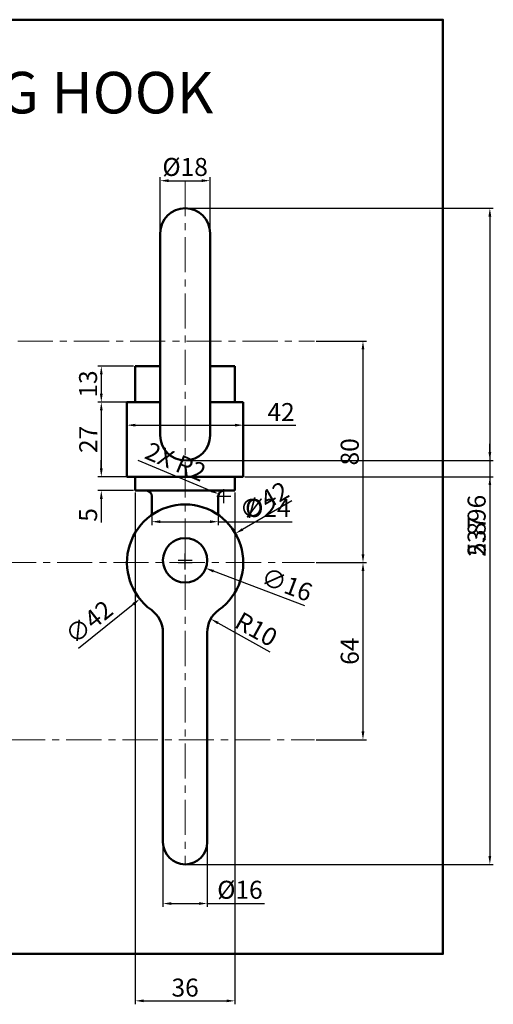
# Model space of a CAD drawing. Units: millimetres. Extents: x 309 to 670, y -17 to 339.
# Tile 2 of 2: x 498 to 670, y -17 to 339. Entities that reach past the tile are written whole.
import ezdxf

# ---------------------------------------------------------------- set-up
doc = ezdxf.new("R2010")
doc.units = ezdxf.units.MM
doc.header["$LTSCALE"] = 0.4
doc.linetypes.add('CENTER', pattern=[50.8, 31.75, -6.35, 6.35, -6.35])
for name, color, linetype, lineweight in [('M-CNTR', 1, 'CENTER', 18), ('M-DIMS', 2, 'Continuous', 25), ('M-OUTL', 7, 'Continuous', 50), ('M-TEXT', 7, 'Continuous', 25), ('M-TTLB', 7, 'Continuous', 50)]:
    doc.layers.add(name, color=color, linetype=linetype, lineweight=lineweight)
doc.styles.get("Standard").update_dxf_attribs({"font": 'arial.ttf'})
doc.dimstyles.new('ISO-25', dxfattribs={"dimtxt": 6.5, "dimasz": 3, "dimexe": 1.25, "dimexo": 0.625, "dimtad": 1, "dimdec": 0, "dimtxsty": 'Standard', "dimcen": 2.5, "dimadec": 0, "dimazin": 0, "dimtfac": 1, "dimtdec": 0, "dimtofl": 0, "dimtmove": 0, "dimatfit": 3, "dimfxl": 1, "dimarcsym": 0})

# ---------------------------------------------------------------- blocks, each defined once
blk = doc.blocks.new('*D1')
at = {"layer": 'Defpoints', "color": 0, "ltscale": 0.4, "transparency": 16777216}
for p in [(540.21, 213.66), (527.93, 200.66), (540.21, 200.66)]:
    blk.add_point(p, dxfattribs=at)
at = {"layer": 'M-DIMS', "color": 0, "lineweight": -2, "ltscale": 0.4, "transparency": 16777216}
for p, q in [((539.58, 213.66), (526.68, 213.66)), ((527.93, 210.66), (527.93, 203.66)), ((539.58, 200.66), (526.68, 200.66))]:
    blk.add_line(p, q, dxfattribs=at)
at = {"layer": 'M-DIMS', "color": 0, "ltscale": 0.4, "transparency": 16777216}
for points in [[(527.43, 210.66), (528.43, 210.66), (527.93, 213.66)], [(527.43, 203.66), (528.43, 203.66), (527.93, 200.66)]]:
    blk.add_solid(points, dxfattribs=at)
at = {"layer": 'M-DIMS', "color": 0, "ltscale": 0.4, "transparency": 16777216, "insert": (523.99, 207.16), "char_height": 6.5, "attachment_point": 5, "rotation": 90}
blk.add_mtext('13', dxfattribs=at)
blk = doc.blocks.new('*D2')
at = {"layer": 'Defpoints', "color": 0, "ltscale": 0.4, "transparency": 16777216}
for p in [(537.21, 200.66), (527.93, 173.66), (537.21, 173.66)]:
    blk.add_point(p, dxfattribs=at)
at = {"layer": 'M-DIMS', "color": 0, "lineweight": -2, "ltscale": 0.4, "transparency": 16777216}
for p, q in [((536.58, 200.66), (526.68, 200.66)), ((527.93, 197.66), (527.93, 176.66)), ((536.58, 173.66), (526.68, 173.66))]:
    blk.add_line(p, q, dxfattribs=at)
at = {"layer": 'M-DIMS', "color": 0, "ltscale": 0.4, "transparency": 16777216}
for points in [[(527.43, 197.66), (528.43, 197.66), (527.93, 200.66)], [(527.43, 176.66), (528.43, 176.66), (527.93, 173.66)]]:
    blk.add_solid(points, dxfattribs=at)
at = {"layer": 'M-DIMS', "color": 0, "ltscale": 0.4, "transparency": 16777216, "insert": (524.05, 187.16), "char_height": 6.5, "attachment_point": 5, "rotation": 90}
blk.add_mtext('27', dxfattribs=at)
blk = doc.blocks.new('*D3')
at = {"layer": 'Defpoints', "color": 0, "ltscale": 0.4, "transparency": 16777216}
for p in [(540.21, 173.66), (527.93, 168.66), (540.21, 168.66)]:
    blk.add_point(p, dxfattribs=at)
at = {"layer": 'M-DIMS', "color": 0, "lineweight": -2, "ltscale": 0.4, "transparency": 16777216}
for p, q in [((527.93, 176.66), (527.93, 179.66)), ((539.58, 173.66), (526.68, 173.66)), ((539.58, 168.66), (526.68, 168.66)), ((527.93, 165.66), (527.93, 157.1))]:
    blk.add_line(p, q, dxfattribs=at)
at = {"layer": 'M-DIMS', "color": 0, "ltscale": 0.4, "transparency": 16777216}
for points in [[(527.43, 176.66), (528.43, 176.66), (527.93, 173.66)], [(527.43, 165.66), (528.43, 165.66), (527.93, 168.66)]]:
    blk.add_solid(points, dxfattribs=at)
at = {"layer": 'M-DIMS', "color": 0, "ltscale": 0.4, "transparency": 16777216, "insert": (524, 159.88), "char_height": 6.5, "attachment_point": 5, "rotation": 90}
blk.add_mtext('5', dxfattribs=at)
blk = doc.blocks.new('*D4')
at = {"layer": 'Defpoints', "color": 0, "ltscale": 0.4, "transparency": 16777216}
for p in [(579.21, 192.3), (537.21, 180.61), (579.21, 180.61)]:
    blk.add_point(p, dxfattribs=at)
at = {"layer": 'M-DIMS', "color": 0, "lineweight": -2, "ltscale": 0.4, "transparency": 16777216}
for p, q in [((537.21, 181.24), (537.21, 193.55)), ((540.21, 192.3), (576.21, 192.3)), ((579.21, 181.24), (579.21, 193.55)), ((579.21, 192.3), (598.25, 192.3))]:
    blk.add_line(p, q, dxfattribs=at)
at = {"layer": 'M-DIMS', "color": 0, "ltscale": 0.4, "transparency": 16777216}
for points in [[(540.21, 192.8), (540.21, 191.8), (537.21, 192.3)], [(576.21, 192.8), (576.21, 191.8), (579.21, 192.3)]]:
    blk.add_solid(points, dxfattribs=at)
at = {"layer": 'M-DIMS', "color": 0, "ltscale": 0.4, "transparency": 16777216, "insert": (592.87, 196.19), "char_height": 6.5, "attachment_point": 5}
blk.add_mtext('42', dxfattribs=at)
blk = doc.blocks.new('*D5')
at = {"layer": 'Defpoints', "color": 0, "ltscale": 0.4, "transparency": 16777216}
for p in [(546.21, 159.89), (570.21, 159.89), (570.21, 157.43)]:
    blk.add_point(p, dxfattribs=at)
at = {"layer": 'M-DIMS', "color": 0, "lineweight": -2, "ltscale": 0.4, "transparency": 16777216}
for p, q in [((546.21, 159.26), (546.21, 156.18)), ((549.21, 157.43), (567.21, 157.43)), ((570.21, 159.26), (570.21, 156.18)), ((570.21, 157.43), (596.93, 157.43))]:
    blk.add_line(p, q, dxfattribs=at)
at = {"layer": 'M-DIMS', "color": 0, "ltscale": 0.4, "transparency": 16777216}
for points in [[(549.21, 157.93), (549.21, 156.93), (546.21, 157.43)], [(567.21, 157.93), (567.21, 156.93), (570.21, 157.43)]]:
    blk.add_solid(points, dxfattribs=at)
at = {"layer": 'M-DIMS', "color": 0, "ltscale": 0.4, "transparency": 16777216, "insert": (588.12, 161.55), "char_height": 6.5, "attachment_point": 5}
blk.add_mtext('%%C24', dxfattribs=at)
blk = doc.blocks.new('*D6')
at = {"layer": 'Defpoints', "color": 0, "ltscale": 0.4, "transparency": 16777216}
for p in [(567.21, 280.61), (549.21, 247.25), (567.21, 247.25)]:
    blk.add_point(p, dxfattribs=at)
at = {"layer": 'M-DIMS', "color": 0, "lineweight": -2, "ltscale": 0.4, "transparency": 16777216}
for p, q in [((549.21, 247.87), (549.21, 281.86)), ((567.21, 247.87), (567.21, 281.86)), ((552.21, 280.61), (564.21, 280.61))]:
    blk.add_line(p, q, dxfattribs=at)
at = {"layer": 'M-DIMS', "color": 0, "ltscale": 0.4, "transparency": 16777216}
for points in [[(552.21, 281.11), (552.21, 280.11), (549.21, 280.61)], [(564.21, 281.11), (564.21, 280.11), (567.21, 280.61)]]:
    blk.add_solid(points, dxfattribs=at)
at = {"layer": 'M-DIMS', "color": 0, "ltscale": 0.4, "transparency": 16777216, "insert": (558.21, 284.73), "char_height": 6.5, "attachment_point": 5}
blk.add_mtext('%%C18', dxfattribs=at)
blk = doc.blocks.new('*D7')
at = {"layer": 'Defpoints', "color": 0, "ltscale": 0.4, "transparency": 16777216}
for p in [(604.93, 222.66), (604.93, 142.66), (622.48, 142.66)]:
    blk.add_point(p, dxfattribs=at)
at = {"layer": 'M-DIMS', "color": 0, "lineweight": -2, "ltscale": 0.4, "transparency": 16777216}
for p, q in [((605.56, 222.66), (623.73, 222.66)), ((622.48, 219.66), (622.48, 145.66)), ((605.56, 142.66), (623.73, 142.66))]:
    blk.add_line(p, q, dxfattribs=at)
at = {"layer": 'M-DIMS', "color": 0, "ltscale": 0.4, "transparency": 16777216}
for points in [[(621.98, 219.66), (622.98, 219.66), (622.48, 222.66)], [(621.98, 145.66), (622.98, 145.66), (622.48, 142.66)]]:
    blk.add_solid(points, dxfattribs=at)
at = {"layer": 'M-DIMS', "color": 0, "ltscale": 0.4, "transparency": 16777216, "insert": (618.53, 182.66), "char_height": 6.5, "attachment_point": 5, "rotation": 90}
blk.add_mtext('80', dxfattribs=at)
blk = doc.blocks.new('*D8')
at = {"layer": 'Defpoints', "color": 0, "ltscale": 0.4, "transparency": 16777216}
for p in [(604.93, 142.66), (604.93, 78.66), (622.48, 78.66)]:
    blk.add_point(p, dxfattribs=at)
at = {"layer": 'M-DIMS', "color": 0, "lineweight": -2, "ltscale": 0.4, "transparency": 16777216}
for p, q in [((605.56, 142.66), (623.73, 142.66)), ((622.48, 139.66), (622.48, 81.66)), ((605.56, 78.66), (623.73, 78.66))]:
    blk.add_line(p, q, dxfattribs=at)
at = {"layer": 'M-DIMS', "color": 0, "ltscale": 0.4, "transparency": 16777216}
for points in [[(621.98, 139.66), (622.98, 139.66), (622.48, 142.66)], [(621.98, 81.66), (622.98, 81.66), (622.48, 78.66)]]:
    blk.add_solid(points, dxfattribs=at)
at = {"layer": 'M-DIMS', "color": 0, "ltscale": 0.4, "transparency": 16777216, "insert": (618.53, 110.66), "char_height": 6.5, "attachment_point": 5, "rotation": 90}
blk.add_mtext('64', dxfattribs=at)
blk = doc.blocks.new('*D9')
at = {"layer": 'Defpoints', "color": 0, "ltscale": 0.4, "transparency": 16777216}
for p in [(550.21, 50.97), (566.21, 50.97), (566.21, 19.51)]:
    blk.add_point(p, dxfattribs=at)
at = {"layer": 'M-DIMS', "color": 0, "lineweight": -2, "ltscale": 0.4, "transparency": 16777216}
for p, q in [((550.21, 50.35), (550.21, 18.26)), ((566.21, 50.35), (566.21, 18.26)), ((553.21, 19.51), (563.21, 19.51)), ((566.21, 19.51), (586.84, 19.51))]:
    blk.add_line(p, q, dxfattribs=at)
at = {"layer": 'M-DIMS', "color": 0, "ltscale": 0.4, "transparency": 16777216}
for points in [[(553.21, 20.01), (553.21, 19.01), (550.21, 19.51)], [(563.21, 20.01), (563.21, 19.01), (566.21, 19.51)]]:
    blk.add_solid(points, dxfattribs=at)
at = {"layer": 'M-DIMS', "color": 0, "ltscale": 0.4, "transparency": 16777216, "insert": (578.02, 23.64), "char_height": 6.5, "attachment_point": 5}
blk.add_mtext('%%C16', dxfattribs=at)
blk = doc.blocks.new('*D10')
at = {"layer": 'Defpoints', "color": 0, "ltscale": 0.4, "transparency": 16777216}
for p in [(567.48, 122.3), (576.21, 117.42)]:
    blk.add_point(p, dxfattribs=at)
at = {"layer": 'M-DIMS', "color": 0, "lineweight": -2, "ltscale": 0.4, "transparency": 16777216}
blk.add_line((588.9, 110.31), (570.1, 120.84), dxfattribs=at)
at = {"layer": 'M-DIMS', "color": 0, "ltscale": 0.4, "transparency": 16777216}
blk.add_solid([(570.34, 121.27), (569.85, 120.4), (567.48, 122.3)], dxfattribs=at)
at = {"layer": 'M-DIMS', "color": 0, "ltscale": 0.4, "transparency": 16777216, "insert": (583.52, 117.85), "char_height": 6.5, "attachment_point": 5, "rotation": 330.7676}
blk.add_mtext('R10', dxfattribs=at)
blk = doc.blocks.new('*D11')
at = {"layer": 'Defpoints', "color": 0, "ltscale": 0.4, "transparency": 16777216}
for p in [(574.59, 155.8), (541.83, 129.51)]:
    blk.add_point(p, dxfattribs=at)
at = {"layer": 'M-DIMS', "color": 0, "lineweight": -2, "ltscale": 0.4, "transparency": 16777216}
for p, q in [((555.71, 142.66), (560.71, 142.66)), ((558.21, 140.16), (558.21, 145.16)), ((519.73, 111.79), (539.49, 127.64))]:
    blk.add_line(p, q, dxfattribs=at)
at = {"layer": 'M-DIMS', "color": 0, "ltscale": 0.4, "transparency": 16777216}
blk.add_solid([(539.17, 128.03), (539.8, 127.25), (541.83, 129.51)], dxfattribs=at)
at = {"layer": 'M-DIMS', "color": 0, "ltscale": 0.4, "transparency": 16777216, "insert": (524, 120.5), "char_height": 6.5, "attachment_point": 5, "rotation": 38.7396}
blk.add_mtext('∅42', dxfattribs=at)
blk = doc.blocks.new('*D12')
at = {"layer": 'Defpoints', "color": 0, "ltscale": 0.4, "transparency": 16777216}
for p in [(550.73, 146.33), (565.68, 140.63)]:
    blk.add_point(p, dxfattribs=at)
at = {"layer": 'M-DIMS', "color": 0, "lineweight": -2, "ltscale": 0.4, "transparency": 16777216}
for p, q in [((558.21, 140.98), (558.21, 145.98)), ((555.71, 143.48), (560.71, 143.48)), ((601.46, 127), (568.49, 139.57))]:
    blk.add_line(p, q, dxfattribs=at)
at = {"layer": 'M-DIMS', "color": 0, "ltscale": 0.4, "transparency": 16777216}
blk.add_solid([(568.66, 140.03), (568.31, 139.1), (565.68, 140.63)], dxfattribs=at)
at = {"layer": 'M-DIMS', "color": 0, "ltscale": 0.4, "transparency": 16777216, "insert": (594.69, 133.99), "char_height": 6.5, "attachment_point": 5, "rotation": 339.135}
blk.add_mtext('∅16', dxfattribs=at)
blk = doc.blocks.new('*D29')
at = {"layer": 'Defpoints', "color": 0, "ltscale": 0.4, "transparency": 16777216}
for p in [(558.21, 270.66), (558.21, 33.66), (668.32, 33.66)]:
    blk.add_point(p, dxfattribs=at)
at = {"layer": 'M-DIMS', "color": 0, "lineweight": -2, "ltscale": 0.4, "transparency": 16777216}
for p, q in [((558.83, 270.66), (669.57, 270.66)), ((668.32, 267.66), (668.32, 36.66)), ((558.83, 33.66), (669.57, 33.66))]:
    blk.add_line(p, q, dxfattribs=at)
at = {"layer": 'M-DIMS', "color": 0, "ltscale": 0.4, "transparency": 16777216}
for points in [[(667.82, 267.66), (668.82, 267.66), (668.32, 270.66)], [(667.82, 36.66), (668.82, 36.66), (668.32, 33.66)]]:
    blk.add_solid(points, dxfattribs=at)
at = {"layer": 'M-DIMS', "color": 0, "ltscale": 0.4, "transparency": 16777216, "insert": (664.37, 152.16), "char_height": 6.5, "attachment_point": 5, "rotation": 90}
blk.add_mtext('237', dxfattribs=at)
blk = doc.blocks.new('*D31')
at = {"layer": 'Defpoints', "color": 0, "ltscale": 0.4, "transparency": 16777216}
for p in [(558.21, 179.55), (579.21, 173.66), (668.32, 173.66)]:
    blk.add_point(p, dxfattribs=at)
at = {"layer": 'M-DIMS', "color": 0, "lineweight": -2, "ltscale": 0.4, "transparency": 16777216}
for p, q in [((668.32, 182.55), (668.32, 185.55)), ((558.83, 179.55), (669.57, 179.55)), ((579.83, 173.66), (669.57, 173.66)), ((668.32, 170.66), (668.32, 144.48))]:
    blk.add_line(p, q, dxfattribs=at)
at = {"layer": 'M-DIMS', "color": 0, "ltscale": 0.4, "transparency": 16777216}
for points in [[(667.82, 182.55), (668.82, 182.55), (668.32, 179.55)], [(667.82, 170.66), (668.82, 170.66), (668.32, 173.66)]]:
    blk.add_solid(points, dxfattribs=at)
at = {"layer": 'M-DIMS', "color": 0, "ltscale": 0.4, "transparency": 16777216, "insert": (664.38, 156.07), "char_height": 6.5, "attachment_point": 5, "rotation": 90}
blk.add_mtext('5.896', dxfattribs=at)
blk = doc.blocks.new('*D32')
at = {"layer": 'Defpoints', "color": 0, "ltscale": 0.4, "transparency": 16777216}
for p in [(540.21, 168.66), (576.21, 168.66), (576.21, -15.64)]:
    blk.add_point(p, dxfattribs=at)
at = {"layer": 'M-DIMS', "color": 0, "lineweight": -2, "ltscale": 0.4, "transparency": 16777216}
for p, q in [((540.21, 168.03), (540.21, -16.89)), ((576.21, 168.03), (576.21, -16.89)), ((543.21, -15.64), (573.21, -15.64))]:
    blk.add_line(p, q, dxfattribs=at)
at = {"layer": 'M-DIMS', "color": 0, "ltscale": 0.4, "transparency": 16777216}
for points in [[(543.21, -15.14), (543.21, -16.14), (540.21, -15.64)], [(573.21, -15.14), (573.21, -16.14), (576.21, -15.64)]]:
    blk.add_solid(points, dxfattribs=at)
at = {"layer": 'M-DIMS', "color": 0, "ltscale": 0.4, "transparency": 16777216, "insert": (558.21, -11.69), "char_height": 6.5, "attachment_point": 5}
blk.add_mtext('36', dxfattribs=at)
blk = doc.blocks.new('*D40')
at = {"layer": 'Defpoints', "color": 0, "ltscale": 0.4, "transparency": 16777216}
for p in [(576.39, 153.16), (540.02, 132.15)]:
    blk.add_point(p, dxfattribs=at)
at = {"layer": 'M-DIMS', "color": 0, "lineweight": -2, "ltscale": 0.4, "transparency": 16777216}
for p, q in [((596.8, 164.95), (578.99, 154.66)), ((555.71, 142.66), (560.71, 142.66)), ((558.21, 140.16), (558.21, 145.16))]:
    blk.add_line(p, q, dxfattribs=at)
at = {"layer": 'M-DIMS', "color": 0, "ltscale": 0.4, "transparency": 16777216}
blk.add_solid([(578.74, 155.09), (579.24, 154.23), (576.39, 153.16)], dxfattribs=at)
at = {"layer": 'M-DIMS', "color": 0, "ltscale": 0.4, "transparency": 16777216, "insert": (587.13, 164.13), "char_height": 6.5, "attachment_point": 5, "rotation": 30.0156}
blk.add_mtext('∅42', dxfattribs=at)
blk = doc.blocks.new('*D41')
at = {"layer": 'Defpoints', "color": 0, "ltscale": 0.4, "transparency": 16777216}
for p in [(570.36, 167.43), (572.21, 166.66)]:
    blk.add_point(p, dxfattribs=at)
at = {"layer": 'M-DIMS', "color": 0, "lineweight": -2, "ltscale": 0.4, "transparency": 16777216}
for p, q in [((541.09, 179.71), (567.6, 168.59)), ((572.21, 164.16), (572.21, 169.16)), ((569.71, 166.66), (574.71, 166.66))]:
    blk.add_line(p, q, dxfattribs=at)
at = {"layer": 'M-DIMS', "color": 0, "ltscale": 0.4, "transparency": 16777216}
blk.add_solid([(567.79, 169.05), (567.4, 168.13), (570.36, 167.43)], dxfattribs=at)
at = {"layer": 'M-DIMS', "color": 0, "ltscale": 0.4, "transparency": 16777216, "insert": (554.47, 178.32), "char_height": 6.5, "attachment_point": 5, "rotation": 337.2422}
blk.add_mtext('2X R2', dxfattribs=at)

msp = doc.modelspace()

# ---------------------------------------------------------------- linework, layer by layer
at = {"layer": 'M-CNTR'}
for p, q in [((558.2071, 280.5288), (558.2071, 33.6555)), ((355.4751, 222.6555), (604.9301, 222.6555)), ((369.74, 142.6555), (604.9301, 142.6555)), ((352.7304, 78.6555), (604.9301, 78.6555))]:
    msp.add_line(p, q, dxfattribs=at)
at = {"layer": 'M-OUTL', "ltscale": 0.4}
for p, q in [((549.2071, 261.6555), (549.2071, 188.5517)), ((567.2071, 261.6555), (567.2071, 188.5517)), ((540.2071, 213.6555), (540.2071, 200.6555)), ((549.2071, 213.6555), (540.2071, 213.6555)), ((576.2071, 213.6555), (567.2071, 213.6555)), ((576.2071, 200.6555), (576.2071, 213.6555)), ((537.2071, 173.6555), (537.2071, 200.6555)), ((537.2071, 200.6555), (549.2071, 200.6555)), ((567.2071, 200.6555), (579.2071, 200.6555)), ((579.2071, 200.6555), (579.2071, 173.6555)), ((579.2071, 173.6555), (537.2071, 173.6555)), ((540.2071, 173.6555), (540.2071, 168.6555)), ((576.2071, 173.6555), (576.2071, 168.6555)), ((576.2071, 168.6555), (540.2071, 168.6555)), ((576.2071, 168.6555), (572.2071, 168.6555)), ((546.2071, 166.6555), (546.2071, 159.8892)), ((570.2071, 166.6555), (570.2071, 159.8892))]:
    msp.add_line(p, q, dxfattribs=at)
at = {"layer": 'M-OUTL'}
for p, q in [((550.2071, 117.4167), (550.2071, 41.6555)), ((566.2071, 117.4167), (566.2071, 41.6555))]:
    msp.add_line(p, q, dxfattribs=at)
msp.add_circle((558.2071, 143.4842), 8, dxfattribs=at)
at = {"layer": 'M-OUTL', "ltscale": 0.4}
for centre, radius, start, end in [((558.2071, 261.6555), 9, 0, 180), ((558.2071, 188.5517), 9, 180, 0), ((544.2071, 166.6555), 2, 0, 90), ((572.2071, 166.6555), 2, 90, 180)]:
    msp.add_arc(centre, radius, start, end, dxfattribs=at)
at = {"layer": 'M-OUTL'}
for centre, radius, start, end in [((558.2071, 142.6555), 21, 305.495933, 234.504067), ((540.2071, 117.4167), 10, 360, 54.504067), ((576.2071, 117.4167), 10, 125.495933, 180), ((558.2071, 41.6555), 8, 180, 0)]:
    msp.add_arc(centre, radius, start, end, dxfattribs=at)
at = {"layer": 'M-TTLB', "ltscale": 0.4}
msp.add_lwpolyline([(333.7348, 338.7612), (651.3692, 338.7612), (651.3692, 1.3112), (333.7348, 1.3112)], close=True, dxfattribs=at)

# ---------------------------------------------------------------- texts
at = {"layer": 'M-TEXT', "ltscale": 0.4, "insert": (429.8042, 319.9085), "char_height": 15, "attachment_point": 1}
msp.add_mtext_dynamic_manual_height_columns('LIFTING HOOK', width=169.632423, gutter_width=12.5, heights=[0], dxfattribs=at)

# ---------------------------------------------------------------- dimensions: what is measured, and where the dimension line sits
at = {"layer": 'M-DIMS', "ltscale": 0.4}
for base, p1, p2, picture, middle in [((567.2071, 280.6082), (549.2071, 247.2468), (567.2071, 247.2468), '*D6', (558.2071, 284.7337)), ((566.2071, 19.5147), (550.2071, 50.9744), (566.2071, 50.9744), '*D9', (578.0214, 23.6403))]:
    dim = msp.add_linear_dim(base=base, p1=p1, p2=p2, text='%%C<>', dimstyle='ISO-25', override={"dimclrd": 0, "dimclre": 0, "dimclrt": 0}, dxfattribs=at)
    dim.commit()
    dim.dimension.update_dxf_attribs({"geometry": picture, "text_midpoint": middle})
for base, p1, p2, override, picture, middle in [((668.3192, 33.6555), (558.2071, 270.6555), (558.2071, 33.6555), {"dimdec": 0, "dimlfac": 1, "dimrnd": 0, "dimzin": 0, "dimdsep": 46, "dimlunit": 2}, '*D29', (664.3732, 152.1555)), ((622.4763, 142.6555), (604.9301, 222.6555), (604.9301, 142.6555), {"dimclrd": 0, "dimclre": 0, "dimclrt": 0}, '*D7', (618.5325, 182.6555)), ((527.9348, 200.6555), (540.2071, 213.6555), (540.2071, 200.6555), {"dimclrd": 0, "dimclre": 0, "dimclrt": 0}, '*D1', (523.9889, 207.1555)), ((527.9348, 173.6555), (537.2071, 200.6555), (537.2071, 173.6555), {"dimclrd": 0, "dimclre": 0, "dimclrt": 0}, '*D2', (524.0465, 187.1555)), ((668.3192, 173.6555), (558.2071, 179.5517), (579.2071, 173.6555), {"dimdec": 3, "dimlfac": 1, "dimrnd": 0, "dimzin": 0, "dimdsep": 46, "dimlunit": 2}, '*D31', (664.3754, 156.0656)), ((527.9348, 168.6555), (540.2071, 173.6555), (540.2071, 168.6555), {"dimclrd": 0, "dimclre": 0, "dimclrt": 0}, '*D3', (524.0044, 159.8757)), ((622.4763, 78.6555), (604.9301, 142.6555), (604.9301, 78.6555), {"dimclrd": 0, "dimclre": 0, "dimclrt": 0}, '*D8', (618.5325, 110.6555))]:
    dim = msp.add_linear_dim(base=base, p1=p1, p2=p2, angle=90, dimstyle='ISO-25', override=override, dxfattribs=at)
    dim.commit()
    dim.dimension.update_dxf_attribs({"geometry": picture, "text_midpoint": middle})
dim = msp.add_linear_dim(base=(579.2071, 192.3017), p1=(537.2071, 180.6119), p2=(579.2071, 180.6119), dimstyle='ISO-25', override={"dimclrd": 0, "dimclre": 0, "dimclrt": 0}, dxfattribs=at)
dim.commit()
dim.dimension.update_dxf_attribs({"geometry": '*D4', "text_midpoint": (592.8731, 192.3017), "dimtype": 160})
dim = msp.add_radius_dim(center=(572.2071, 166.6555), mpoint=(570.3629, 167.4292), text='2X <>', dimstyle='ISO-25', override={"dimdec": 0, "dimlfac": 1, "dimrnd": 0, "dimzin": 0, "dimdsep": 46, "dimlunit": 2}, dxfattribs=at)
dim.commit()
dim.dimension.update_dxf_attribs({"geometry": '*D41', "text_midpoint": (554.4658, 178.3169)})
for p1, p2, override, picture, middle in [((540.0235, 132.1506), (576.3908, 153.1605), {"dimdec": 0, "dimlfac": 1, "dimrnd": 0, "dimzin": 0, "dimdsep": 46, "dimlunit": 2}, '*D40', (589.1915, 160.5556)), ((574.5871, 155.7969), (541.8272, 129.5141), {"dimclrd": 0, "dimclre": 0, "dimclrt": 0}, '*D11', (526.5807, 117.282)), ((550.7318, 146.3336), (565.6825, 140.6349), {"dimclrd": 0, "dimclre": 0, "dimclrt": 0}, '*D12', (593.2241, 130.1371))]:
    dim = msp.add_diameter_dim_2p(p1=p1, p2=p2, dimstyle='ISO-25', override=override, dxfattribs=at)
    dim.commit()
    dim.dimension.update_dxf_attribs({"geometry": picture, "text_midpoint": middle, "dimtype": 163})
dim = msp.add_linear_dim(base=(576.2071, -15.6388), p1=(540.2071, 168.6555), p2=(576.2071, 168.6555), dimstyle='ISO-25', override={"dimdec": 0, "dimlfac": 1, "dimrnd": 0, "dimzin": 0, "dimdsep": 46, "dimlunit": 2}, dxfattribs=at)
dim.commit()
dim.dimension.update_dxf_attribs({"geometry": '*D32', "text_midpoint": (558.2071, -11.6929)})
dim = msp.add_linear_dim(base=(570.2071, 157.4288), p1=(546.2071, 159.8892), p2=(570.2071, 159.8892), text='%%C<>', dimstyle='ISO-25', override={"dimclrd": 0, "dimclre": 0, "dimclrt": 0}, dxfattribs=at)
dim.commit()
dim.dimension.update_dxf_attribs({"geometry": '*D5', "text_midpoint": (588.1219, 157.4288), "dimtype": 160})
dim = msp.add_radius_dim(center=(576.2071, 117.4167), mpoint=(567.4807, 122.3002), dimstyle='ISO-25', override={"dimclrd": 0, "dimclre": 0, "dimclrt": 0}, dxfattribs=at)
dim.commit()
dim.dimension.update_dxf_attribs({"geometry": '*D10', "text_midpoint": (581.5908, 114.4038), "dimtype": 164})

doc.saveas('drawing.dxf')
